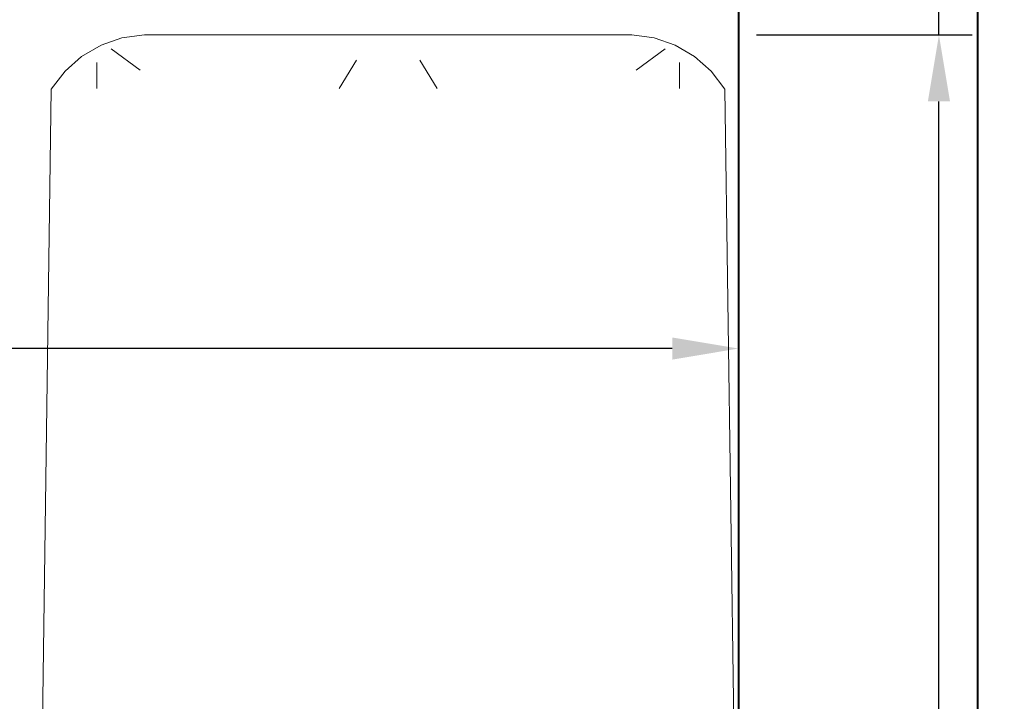
# Model space of a CAD drawing. Units: inches. Extents: x 2337 to 3570, y 1258 to 1938.
# Tile 11 of 30: x 2837 to 2874, y 1651 to 1677. Entities that reach past the tile are written whole.
import ezdxf

# ---------------------------------------------------------------- set-up
doc = ezdxf.new("R2010")
doc.units = ezdxf.units.IN
for name, color, linetype, lineweight in [('A-ANNO-DIMS', 2, 'Continuous', 18), ('A-WALL', 7, 'Continuous', 40), ('furn', 8, 'Continuous', 18)]:
    doc.layers.add(name, color=color, linetype=linetype, lineweight=lineweight)
doc.styles.get("Standard").update_dxf_attribs({"font": 'arial.ttf'})
doc.dimstyles.new('ISO-25', dxfattribs={"dimtxt": 9, "dimasz": 2.5, "dimexe": 1.25, "dimexo": 0.625, "dimtad": 1, "dimdec": 1, "dimlunit": 3, "dimtxsty": 'Standard', "dimcen": 2.5, "dimadec": 0, "dimazin": 0, "dimtfac": 1, "dimtdec": 1, "dimtmove": 0, "dimatfit": 3, "dimfxl": 1, "dimarcsym": 0})

# ---------------------------------------------------------------- blocks, each defined once
blk = doc.blocks.new('sofa-49')
at = {"color": 0, "linetype": 'ByBlock'}
for p, q in [((-0.0945, 1.6514), (-0.1206, 1.6424)), ((-0.0945, 1.6514), (-0.1206, 1.6424)), ((-0.0666, 1.655), (-0.0945, 1.6514)), ((-0.0666, 1.655), (-0.0945, 1.6514)), ((0.2376, 1.655), (-0.0666, 1.655)), ((0.2376, 1.655), (-0.0666, 1.655)), ((0.5418, 1.655), (0.2376, 1.655)), ((0.5418, 1.655), (0.2376, 1.655)), ((0.5697, 1.6514), (0.5418, 1.655)), ((0.5697, 1.6514), (0.5418, 1.655)), ((0.5958, 1.6424), (0.5697, 1.6514)), ((0.5958, 1.6424), (0.5697, 1.6514)), ((-0.1206, 1.6424), (-0.1449, 1.628)), ((-0.1206, 1.6424), (-0.1449, 1.628)), ((-0.072, 1.6109), (-0.108, 1.6379)), ((0.5472, 1.6109), (0.5832, 1.6379)), ((0.6201, 1.628), (0.5958, 1.6424)), ((0.6201, 1.628), (0.5958, 1.6424)), ((-0.1449, 1.628), (-0.1656, 1.61)), ((-0.1449, 1.628), (-0.1656, 1.61)), ((0.1764, 1.5884), (0.198, 1.6235)), ((0.2772, 1.6235), (0.2988, 1.5884)), ((0.6408, 1.61), (0.6201, 1.628)), ((0.6408, 1.61), (0.6201, 1.628)), ((-0.1656, 1.61), (-0.1827, 1.5875)), ((-0.1656, 1.61), (-0.1827, 1.5875)), ((-0.126, 1.6208), (-0.126, 1.5884)), ((0.6012, 1.6208), (0.6012, 1.5884)), ((0.6579, 1.5875), (0.6408, 1.61)), ((0.6579, 1.5875), (0.6408, 1.61)), ((-0.1827, 1.5875), (-0.1944, 0.7614)), ((-0.1827, 1.5875), (-0.1944, 0.7614)), ((0.6696, 0.7614), (0.6579, 1.5875)), ((0.6696, 0.7614), (0.6579, 1.5875)), ((-0.1944, 0.7614), (-0.2007, 0.7344)), ((-0.1944, 0.7614), (-0.2007, 0.7344)), ((0.6759, 0.7344), (0.6696, 0.7614)), ((0.6759, 0.7344), (0.6696, 0.7614)), ((-0.1872, 0.7326), (-0.1791, 0.738)), ((-0.1791, 0.738), (-0.1692, 0.7407)), ((-0.1692, 0.7407), (-0.1593, 0.7416)), ((-0.1593, 0.7416), (-0.0486, 0.7416)), ((-0.0486, 0.7416), (-0.0378, 0.7416)), ((-0.0378, 0.7416), (-0.0279, 0.7389)), ((-0.0279, 0.7389), (-0.0189, 0.7335)), ((0.4941, 0.7335), (0.5031, 0.7389)), ((0.5031, 0.7389), (0.513, 0.7416)), ((0.513, 0.7416), (0.5238, 0.7416)), ((0.5238, 0.7416), (0.6345, 0.7416)), ((0.6345, 0.7416), (0.6444, 0.7407)), ((0.6444, 0.7407), (0.6543, 0.738)), ((0.6543, 0.738), (0.6624, 0.7326)), ((-0.2007, 0.7344), (-0.2016, 0.7065)), ((-0.2007, 0.7344), (-0.2016, 0.7065)), ((-0.1989, 0.7164), (-0.1944, 0.7254)), ((-0.1944, 0.7254), (-0.1872, 0.7326)), ((-0.0189, 0.7335), (-0.0117, 0.7263)), ((-0.0117, 0.7263), (-0.0063, 0.7182)), ((0.4815, 0.7182), (0.4869, 0.7263)), ((0.4869, 0.7263), (0.4941, 0.7335)), ((0.6624, 0.7326), (0.6696, 0.7254)), ((0.6696, 0.7254), (0.6741, 0.7164)), ((0.6768, 0.7065), (0.6759, 0.7344)), ((0.6768, 0.7065), (0.6759, 0.7344)), ((-0.2016, 0.7065), (-0.1989, 0.7164)), ((-0.0351, 0.7074), (-0.0324, 0.72)), ((-0.0063, 0.7182), (-0.0027, 0.7083)), ((0.4779, 0.7083), (0.4815, 0.7182)), ((0.5103, 0.7074), (0.5076, 0.72)), ((0.6741, 0.7164), (0.6768, 0.7065)), ((-0.2016, 0.2034), (-0.2016, 0.7065)), ((-0.2016, 0.7065), (-0.2016, 0.2034)), ((-0.0351, 0.7029), (-0.0126, 0.7074)), ((-0.0027, 0.7083), (-0.0027, 0.6975)), ((0.0099, 0.6462), (-0.0027, 0.7083)), ((0.4779, 0.7083), (0.4599, 0.6372)), ((0.4779, 0.6975), (0.4779, 0.7083)), ((0.5103, 0.7029), (0.4878, 0.7074)), ((0.6768, 0.7065), (0.6768, 0.2034)), ((0.6768, 0.2034), (0.6768, 0.7065)), ((-0.1746, 0.693), (-0.162, 0.693)), ((-0.1431, 0.693), (-0.126, 0.693)), ((-0.1035, 0.693), (-0.0864, 0.693)), ((-0.072, 0.693), (-0.054, 0.693)), ((-0.0396, 0.693), (-0.0396, 0.639)), ((-0.0027, 0.6975), (-0.0027, 0.2034)), ((0.4779, 0.2034), (0.4779, 0.6975)), ((0.5148, 0.693), (0.5148, 0.639)), ((0.5472, 0.693), (0.5292, 0.693)), ((0.5787, 0.693), (0.5616, 0.693)), ((0.6183, 0.693), (0.6012, 0.693)), ((0.6498, 0.693), (0.6372, 0.693)), ((0.0198, 0.5832), (0.0099, 0.6462)), ((0.4599, 0.6372), (0.4473, 0.5652)), ((-0.0396, 0.585), (-0.0396, 0.558)), ((0.0252, 0.5193), (0.0198, 0.5832)), ((0.5148, 0.585), (0.5148, 0.558)), ((0.4473, 0.5652), (0.441, 0.4923)), ((0.027, 0.4554), (0.0252, 0.5193)), ((-0.0396, 0.4077), (-0.0396, 0.5067)), ((0.5148, 0.4077), (0.5148, 0.5067)), ((0.441, 0.4923), (0.441, 0.4194)), ((0.0252, 0.3924), (0.027, 0.4554)), ((0.441, 0.4194), (0.4473, 0.3465)), ((0.0198, 0.3285), (0.0252, 0.3924)), ((-0.0396, 0.3267), (-0.0396, 0.3537)), ((0.4473, 0.3465), (0.4599, 0.2745)), ((0.5148, 0.3267), (0.5148, 0.3537)), ((0.4167, 0.3015), (0.4104, 0.3402)), ((0.0108, 0.2655), (0.0198, 0.3285)), ((0.0531, 0.2826), (0.0621, 0.3186)), ((0.0855, 0.2907), (0.1116, 0.3015)), ((0.4104, 0.2781), (0.3969, 0.2934)), ((0.1683, 0.2718), (0.1233, 0.2619)), ((0.2142, 0.2763), (0.1683, 0.2718)), ((0.261, 0.2763), (0.2142, 0.2763)), ((0.3069, 0.2718), (0.261, 0.2763)), ((0.3519, 0.2619), (0.3069, 0.2718)), ((0.4599, 0.2745), (0.4779, 0.2034)), ((-0.0027, 0.2034), (0.0108, 0.2655)), ((0.1233, 0.2619), (0.0792, 0.2466)), ((0.396, 0.2466), (0.3519, 0.2619)), ((0.0792, 0.2466), (0.0369, 0.2277)), ((0.4383, 0.2277), (0.396, 0.2466)), ((-0.0396, 0.2187), (-0.0396, 0.2358)), ((0.5148, 0.2187), (0.5148, 0.2358)), ((0.0369, 0.2277), (-0.0027, 0.2034)), ((0.4779, 0.2034), (0.4383, 0.2277)), ((-0.1998, 0.1746), (-0.2016, 0.2034)), ((-0.2016, 0.2034), (-0.1998, 0.1746)), ((-0.0765, 0.1152), (-0.0045, 0.2016)), ((-0.0045, 0.2016), (-0.0711, 0.135)), ((-0.0027, 0.2034), (0.2376, 0.2034)), ((0.2376, 0.2034), (0.4779, 0.2034)), ((0.5463, 0.135), (0.4797, 0.2016)), ((0.4797, 0.2016), (0.5517, 0.1152)), ((0.6768, 0.2034), (0.675, 0.1746)), ((0.675, 0.1746), (0.6768, 0.2034)), ((-0.1935, 0.1458), (-0.1998, 0.1746)), ((-0.1998, 0.1746), (-0.1935, 0.1458)), ((0.675, 0.1746), (0.6687, 0.1458)), ((0.6687, 0.1458), (0.675, 0.1746)), ((-0.0324, 0.1647), (0.0216, 0.1647)), ((0.0756, 0.1647), (0.1026, 0.1647)), ((0.1566, 0.1647), (0.2106, 0.1647)), ((0.3186, 0.1647), (0.2646, 0.1647)), ((0.3996, 0.1647), (0.3726, 0.1647)), ((0.5076, 0.1647), (0.4536, 0.1647)), ((-0.1836, 0.1188), (-0.1935, 0.1458)), ((-0.1935, 0.1458), (-0.1836, 0.1188)), ((0.6687, 0.1458), (0.6588, 0.1188)), ((0.6588, 0.1188), (0.6687, 0.1458)), ((-0.0711, 0.135), (-0.0927, 0.1197)), ((0.5679, 0.1197), (0.5463, 0.135)), ((-0.1701, 0.0936), (-0.1836, 0.1188)), ((-0.1836, 0.1188), (-0.1701, 0.0936)), ((-0.0927, 0.1197), (-0.1152, 0.1062)), ((-0.09, 0.0972), (-0.0765, 0.1152)), ((0.5517, 0.1152), (0.5652, 0.0972)), ((0.5904, 0.1062), (0.5679, 0.1197)), ((0.6588, 0.1188), (0.6453, 0.0936)), ((0.6453, 0.0936), (0.6588, 0.1188)), ((-0.1152, 0.1062), (-0.1395, 0.0954)), ((0.6147, 0.0954), (0.5904, 0.1062)), ((-0.153, 0.0702), (-0.1701, 0.0936)), ((-0.1701, 0.0936), (-0.153, 0.0702)), ((-0.1395, 0.0954), (-0.1647, 0.0873)), ((-0.0999, 0.0774), (-0.09, 0.0972)), ((0.5652, 0.0972), (0.5751, 0.0774)), ((0.6399, 0.0873), (0.6147, 0.0954)), ((0.6453, 0.0936), (0.6282, 0.0702)), ((0.6282, 0.0702), (0.6453, 0.0936)), ((-0.1062, 0.0558), (-0.0999, 0.0774)), ((0.5751, 0.0774), (0.5814, 0.0558)), ((-0.1323, 0.0495), (-0.153, 0.0702)), ((-0.153, 0.0702), (-0.1323, 0.0495)), ((0.6282, 0.0702), (0.6075, 0.0495)), ((0.6075, 0.0495), (0.6282, 0.0702)), ((-0.1098, 0.0324), (-0.1323, 0.0495)), ((-0.1323, 0.0495), (-0.1082, 0.0312)), ((-0.108, 0.0333), (-0.1062, 0.0558)), ((0.5814, 0.0558), (0.5832, 0.0333)), ((0.6075, 0.0495), (0.585, 0.0324)), ((0.585, 0.0324), (0.6075, 0.0495)), ((-0.0846, 0.018), (-0.1098, 0.0324)), ((-0.1082, 0.0312), (-0.1081, 0.0315)), ((-0.1081, 0.0315), (-0.0846, 0.018)), ((0.585, 0.0324), (0.5598, 0.018)), ((0.5598, 0.018), (0.585, 0.0324)), ((-0.0567, 0.0081), (-0.0846, 0.018)), ((-0.0846, 0.018), (-0.0567, 0.0081)), ((0.5598, 0.018), (0.5319, 0.0081)), ((0.5319, 0.0081), (0.5598, 0.018)), ((-0.0288, 0.0018), (-0.0567, 0.0081)), ((-0.0567, 0.0081), (-0.0288, 0.0018)), ((0, 0), (-0.0288, 0.0018)), ((-0.0288, 0.0018), (0, 0)), ((0.2376, 0), (0, 0)), ((0, 0), (0.2376, 0)), ((0.4752, 0), (0.2376, 0)), ((0.2376, 0), (0.4752, 0)), ((0.504, 0.0018), (0.4752, 0)), ((0.4752, 0), (0.504, 0.0018)), ((0.5319, 0.0081), (0.504, 0.0018)), ((0.504, 0.0018), (0.5319, 0.0081))]:
    blk.add_line(p, q, dxfattribs=at)
blk = doc.blocks.new('*D86')
at = {"layer": 'A-ANNO-DIMS', "color": 0, "lineweight": -2, "transparency": 16777216}
for p, q in [((2762.092, 1679.329), (2762.092, 1663.443)), ((2863.836, 1679.329), (2863.836, 1663.443)), ((2762.092, 1664.693), (2617.848, 1664.693)), ((2861.336, 1664.693), (2764.592, 1664.693))]:
    blk.add_line(p, q, dxfattribs=at)
at = {"layer": 'A-ANNO-DIMS', "color": 0, "transparency": 16777216}
for points in [[(2764.592, 1665.109), (2764.592, 1664.276), (2762.092, 1664.693)], [(2861.336, 1665.109), (2861.336, 1664.276), (2863.836, 1664.693)]]:
    blk.add_solid(points, dxfattribs=at)
at = {"layer": 'Defpoints', "color": 0, "transparency": 16777216}
for p in [(2762.092, 1679.954), (2863.836, 1679.954), (2762.092, 1664.693)]:
    blk.add_point(p, dxfattribs=at)
at = {"layer": 'A-ANNO-DIMS', "color": 0, "transparency": 16777216, "insert": (2688.72, 1669.974), "char_height": 9, "attachment_point": 5}
blk.add_mtext('CORNER SOFA 8\'-5 1/2"', dxfattribs=at)
blk = doc.blocks.new('*D90')
at = {"layer": 'A-ANNO-DIMS', "color": 0, "lineweight": -2, "transparency": 16777216}
for p, q in [((2871.382, 1676.497), (2871.382, 1796.695)), ((2864.515, 1676.497), (2872.632, 1676.497)), ((2871.382, 1629.048), (2871.382, 1673.997)), ((2864.515, 1626.548), (2872.632, 1626.548))]:
    blk.add_line(p, q, dxfattribs=at)
at = {"layer": 'A-ANNO-DIMS', "color": 0, "transparency": 16777216}
for points in [[(2870.966, 1673.997), (2871.799, 1673.997), (2871.382, 1676.497)], [(2870.966, 1629.048), (2871.799, 1629.048), (2871.382, 1626.548)]]:
    blk.add_solid(points, dxfattribs=at)
at = {"layer": 'Defpoints', "color": 0, "transparency": 16777216}
for p in [(2863.89, 1676.497), (2871.382, 1676.497), (2863.89, 1626.548)]:
    blk.add_point(p, dxfattribs=at)
at = {"layer": 'A-ANNO-DIMS', "color": 0, "transparency": 16777216, "insert": (2866.101, 1737.846), "char_height": 9, "attachment_point": 5, "rotation": 90}
blk.add_mtext('LOUNGE SEAT 4\'-2"', dxfattribs=at)

msp = doc.modelspace()

# ---------------------------------------------------------------- linework, layer by layer
at = {"layer": 'A-WALL'}
for p, q in [((2872.836, 1764.116), (2872.836, 1542.116)), ((2863.836, 1755.116), (2863.836, 1551.116))]:
    msp.add_line(p, q, dxfattribs=at)

# ---------------------------------------------------------------- block references
at = {"layer": 'furn', "xscale": 30.18064521598093, "yscale": 30.18064521598093, "zscale": 30.18064521598093}
msp.add_blockref('sofa-49', (2843.464, 1626.548), dxfattribs=at)

# ---------------------------------------------------------------- dimensions: what is measured, and where the dimension line sits
at = {"layer": 'A-ANNO-DIMS'}
for base, p1, p2, angle, text, picture, middle in [((2871.382, 1676.497), (2863.89, 1626.548), (2863.89, 1676.497), 90, 'LOUNGE SEAT <>', '*D90', (2866.101, 1737.846)), ((2762.092, 1664.693), (2863.836, 1679.954), (2762.092, 1679.954), 180, 'CORNER SOFA <>', '*D86', (2688.72, 1669.974))]:
    dim = msp.add_linear_dim(base=base, p1=p1, p2=p2, angle=angle, text=text, dimstyle='ISO-25', override={"dimdec": 1, "dimlfac": 1, "dimrnd": 0, "dimzin": 1, "dimdsep": 46, "dimlunit": 4, "dimfrac": 2}, dxfattribs=at)
    dim.commit()
    dim.dimension.update_dxf_attribs({"geometry": picture, "text_midpoint": middle})

doc.saveas('drawing.dxf')
